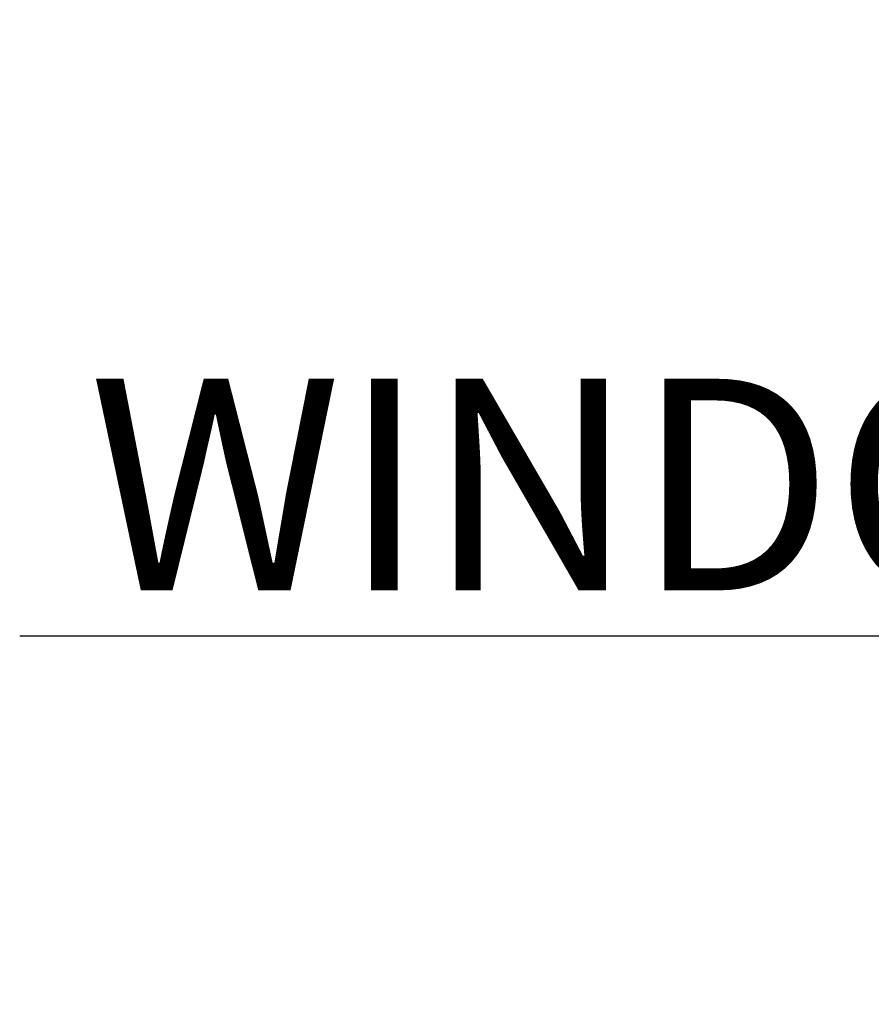
# Model space of a CAD drawing. Units: inches. Extents: x 3148 to 3962, y 1142 to 1671.
# Tile 7 of 9: x 3519 to 3555, y 1507 to 1549. Entities that reach past the tile are written whole.
import ezdxf

# ---------------------------------------------------------------- set-up
doc = ezdxf.new("R2010")
doc.units = ezdxf.units.IN
doc.layers.add('A-ANNO-DIMS', color=2, linetype='Continuous', lineweight=18)
doc.styles.get("Standard").update_dxf_attribs({"font": 'arial.ttf'})
doc.dimstyles.new('ISO-25', dxfattribs={"dimtxt": 9, "dimasz": 2.5, "dimexe": 1.25, "dimexo": 0.625, "dimtad": 1, "dimdec": 1, "dimlunit": 3, "dimtxsty": 'Standard', "dimcen": 2.5, "dimadec": 0, "dimazin": 0, "dimtfac": 1, "dimtdec": 1, "dimtmove": 0, "dimatfit": 3, "dimfxl": 1, "dimarcsym": 0})

# ---------------------------------------------------------------- blocks, each defined once
blk = doc.blocks.new('*D72')
at = {"layer": 'A-ANNO-DIMS', "color": 0, "lineweight": -2, "transparency": 16777216}
for p, q in [((3636.331, 1519.424), (3636.331, 1523.649)), ((3660.331, 1519.424), (3660.331, 1523.649)), ((3636.331, 1522.399), (3518.693, 1522.399)), ((3657.831, 1522.399), (3638.831, 1522.399))]:
    blk.add_line(p, q, dxfattribs=at)
at = {"layer": 'A-ANNO-DIMS', "color": 0, "transparency": 16777216}
for points in [[(3638.831, 1522.816), (3638.831, 1521.983), (3636.331, 1522.399)], [(3657.831, 1522.816), (3657.831, 1521.983), (3660.331, 1522.399)]]:
    blk.add_solid(points, dxfattribs=at)
at = {"layer": 'Defpoints', "color": 0, "transparency": 16777216}
for p in [(3636.331, 1522.399), (3636.331, 1518.799), (3660.331, 1518.799)]:
    blk.add_point(p, dxfattribs=at)
at = {"layer": 'A-ANNO-DIMS', "color": 0, "transparency": 16777216, "insert": (3576.262, 1527.681), "char_height": 9, "attachment_point": 5}
blk.add_mtext('WINDOW 2\'-0" TYP.', dxfattribs=at)

msp = doc.modelspace()

# ---------------------------------------------------------------- dimensions: what is measured, and where the dimension line sits
at = {"layer": 'A-ANNO-DIMS'}
dim = msp.add_linear_dim(base=(3636.331, 1522.399), p1=(3660.331, 1518.799), p2=(3636.331, 1518.799), angle=180, text='WINDOW <> TYP.', dimstyle='ISO-25', override={"dimdec": 1, "dimlfac": 1, "dimrnd": 0, "dimzin": 1, "dimdsep": 46, "dimlunit": 4, "dimfrac": 2}, dxfattribs=at)
dim.commit()
dim.dimension.update_dxf_attribs({"geometry": '*D72', "text_midpoint": (3576.262, 1527.681)})

doc.saveas('drawing.dxf')
